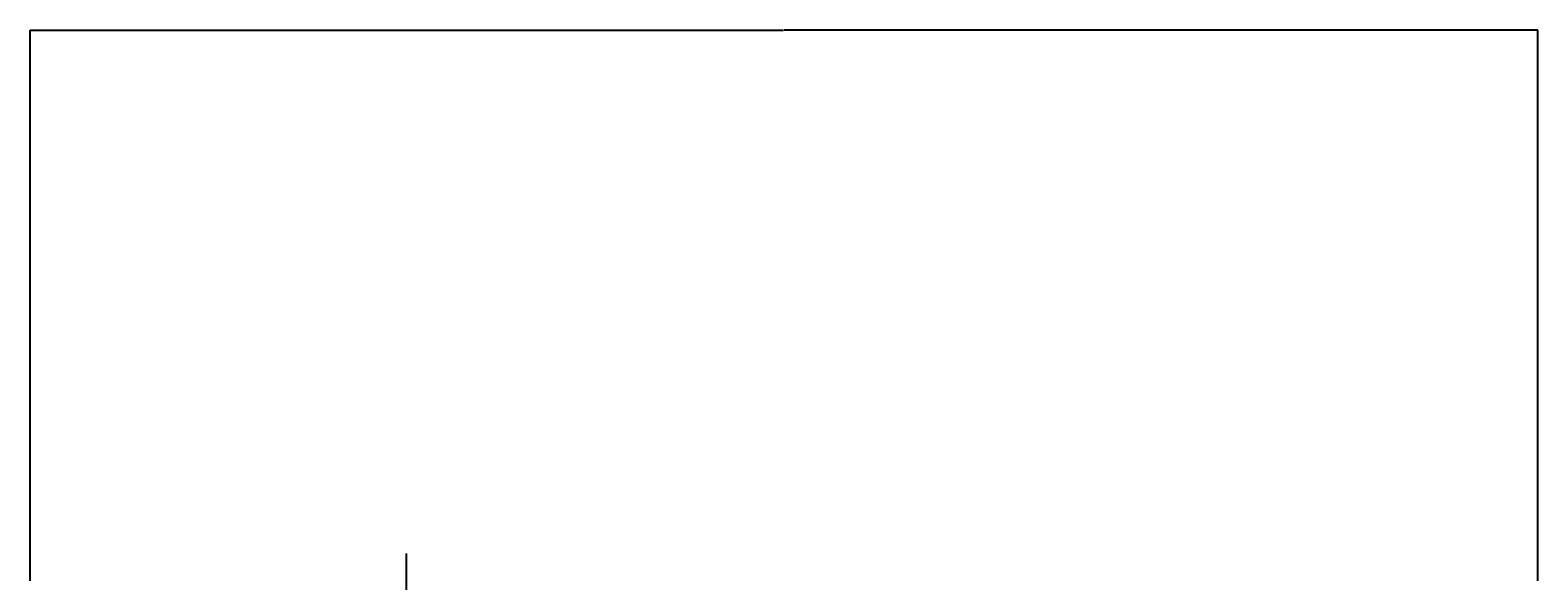
# Model space of a CAD drawing. Units: millimetres. Extents: x 756 to 17937, y 31 to 15590.
# Tile 6 of 6: x 14792 to 16791, y 7660 to 8390. Entities that reach past the tile are written whole.
import ezdxf

# ---------------------------------------------------------------- set-up
doc = ezdxf.new("R2010")
doc.units = ezdxf.units.MM
doc.layers.add('A-ANNO-DIMS', color=2, linetype='Continuous', lineweight=18)
doc.layers.add('A-FLOR-STRS', color=7, linetype='Continuous', lineweight=25)
doc.styles.get("Standard").update_dxf_attribs({"font": 'arial.ttf'})
doc.dimstyles.get("Standard").update_dxf_attribs({"dimtxt": 0.18, "dimasz": 0.18, "dimexe": 0.18, "dimexo": 0.0625, "dimgap": 0.09, "dimtad": 0, "dimtih": 1, "dimtoh": 1, "dimdec": 4, "dimzin": 0, "dimdsep": 46, "dimtxsty": 'Standard', "dimcen": 0.09, "dimadec": 0, "dimazin": 0, "dimtfac": 1, "dimtdec": 4, "dimtofl": 0, "dimtmove": 0, "dimatfit": 3, "dimfxl": 1, "dimtolj": 1, "dimtzin": 0, "dimarcsym": 0})

# ---------------------------------------------------------------- blocks, each defined once
blk = doc.blocks.new('*D58')
at = {"layer": 'A-ANNO-DIMS', "color": 0, "lineweight": -2, "transparency": 16777216}
for p, q in [((14792.2, 7660.2), (14792.2, 8389.6)), ((14792.4, 8389.4), (15791.1, 8389.4)), ((16790.7, 8389.4), (15792, 8389.4)), ((16790.9, 7660.2), (16790.9, 8389.6))]:
    blk.add_line(p, q, dxfattribs=at)
at = {"layer": 'A-ANNO-DIMS', "color": 0, "transparency": 16777216}
for points in [[(14792.4, 8389.4), (14792.4, 8389.4), (14792.2, 8389.4)], [(16790.7, 8389.4), (16790.7, 8389.4), (16790.9, 8389.4)]]:
    blk.add_solid(points, dxfattribs=at)
at = {"layer": 'Defpoints', "color": 0, "transparency": 16777216}
for p in [(16790.9, 8389.4), (14792.2, 7660.2), (16790.9, 7660.2)]:
    blk.add_point(p, dxfattribs=at)
at = {"layer": 'A-ANNO-DIMS', "color": 0, "transparency": 16777216, "insert": (15791.6, 8389.4), "char_height": 0.18, "attachment_point": 5}
blk.add_mtext('\\A1;1998.7', dxfattribs=at)

msp = doc.modelspace()

# ---------------------------------------------------------------- linework, layer by layer
at = {"layer": 'A-FLOR-STRS'}
msp.add_line((15290.928, 6900.77), (15290.928, 7696.562), dxfattribs=at)

# ---------------------------------------------------------------- dimensions: what is measured, and where the dimension line sits
at = {"layer": 'A-ANNO-DIMS'}
dim = msp.add_linear_dim(base=(16790.928, 8389.41), p1=(14792.241, 7660.16), p2=(16790.928, 7660.16), angle=0, dimstyle='Standard', override={"dimdec": 1, "dimlfac": 1, "dimrnd": 0, "dimzin": 0, "dimdsep": 46, "dimlunit": 2}, dxfattribs=at)
dim.commit()
dim.dimension.update_dxf_attribs({"geometry": '*D58', "text_midpoint": (15791.585, 8389.41)})

doc.saveas('drawing.dxf')
